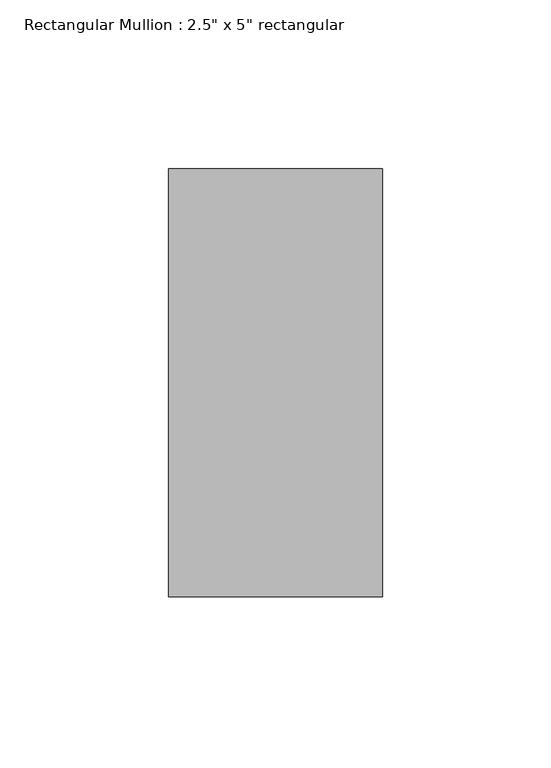
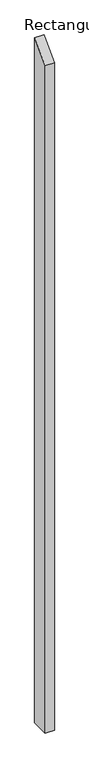
"""IFC4 building model written with IfcOpenShell, lengths in millimetres: member geometry."""

from ifc_helpers import new_model, si_unit, frame, origin, place, context, project, spatial, polyline, outline, extrude, source, transform, mapped, element, save


def member_d319704e(model_context):
    return source(origin(), model_context, "Body", "SweptSolid", [
        extrude(outline(polyline([(-63.5, -63.5), (63.5, 63.5), (63.5, -4976.9981466), (-63.5, -4976.9981466), (-63.5, -63.5)])), frame((-63.5, 0.0, 0.0), z_axis=(1.0, 0.0, 0.0), x_axis=(0.0, 1.0, 0.0)), (0.0, 0.0, 1.0), 63.5),
    ])


if __name__ == "__main__":
    model = new_model("IFC4")
    model_context = context("Model", 3, world=origin())
    ifc_project = project(units=[si_unit("LENGTHUNIT", "METRE", prefix="MILLI")], contexts=[model_context])
    site = spatial("IfcSite", under=ifc_project)
    building = spatial("IfcBuilding", under=site)
    placement = place(None, origin())
    member_shape = member_d319704e(model_context)
    element("IfcMember", 1, ObjectType="Rectangular Mullion : 2.5\" x 5\" rectangular", at=placement, inside=building, context=model_context, shape_type="MappedRepresentation", body=[
        mapped(member_shape, transform((0.0, 0.0, 0.0), x_axis=(1.0, 0.0, 0.0), y_axis=(0.0, 1.0, 0.0), z_axis=(0.0, 0.0, 1.0))),
    ])
    save(model, "model.ifc")

# Revit data of these elements
# Type "Rectangular Mullion : 2.5\" x 5\" rectangular"
#   built-in parameter 1007304 = 0.416667 (stored number, unit not read)
#   built-in parameter 1007301 = 0.104167 (stored number, unit not read)
#   built-in parameter 1007300 = 0.104167 (stored number, unit not read)
# Element 1 (IfcMember, "Rectangular Mullion : 2.5\" x 5\" rectangular")
#   Materials on its faces: "Aluminum"
# Materials
#   "Aluminum": class "Metal", colour RGB 247 247 247, transparency 0, Description = "Aluminum 6061", Cost = 0
